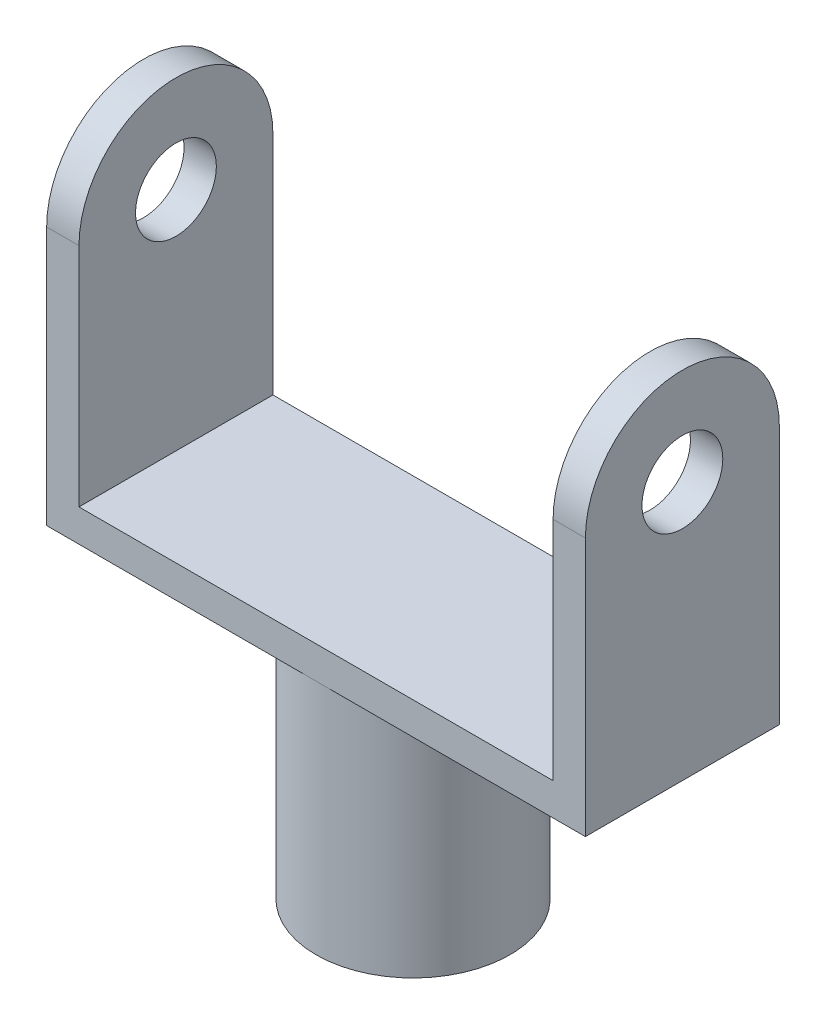
ISO-10303-21;
HEADER;
FILE_DESCRIPTION(('STEP AP214'),'2;1');
FILE_NAME('part.step','',(''),(''),'','','');
FILE_SCHEMA(('AUTOMOTIVE_DESIGN { 1 0 10303 214 1 1 1 1 }'));
ENDSEC;
DATA;
#1=APPLICATION_CONTEXT('core data for automotive mechanical design processes');
#2=APPLICATION_PROTOCOL_DEFINITION('international standard','automotive_design',2000,#1);
#3=PRODUCT_CONTEXT('',#1,'mechanical');
#4=PRODUCT('Part','Part','',(#3));
#5=PRODUCT_RELATED_PRODUCT_CATEGORY('part','',(#4));
#6=PRODUCT_DEFINITION_FORMATION('','',#4);
#7=PRODUCT_DEFINITION_CONTEXT('part definition',#1,'design');
#8=PRODUCT_DEFINITION('design','',#6,#7);
#9=PRODUCT_DEFINITION_SHAPE('','',#8);
#10=(LENGTH_UNIT() NAMED_UNIT(*) SI_UNIT(.MILLI.,.METRE.));
#11=(NAMED_UNIT(*) PLANE_ANGLE_UNIT() SI_UNIT($,.RADIAN.));
#12=(NAMED_UNIT(*) SI_UNIT($,.STERADIAN.) SOLID_ANGLE_UNIT());
#13=UNCERTAINTY_MEASURE_WITH_UNIT(LENGTH_MEASURE(1.E-05),#10,'distance_accuracy_value','');
#14=(GEOMETRIC_REPRESENTATION_CONTEXT(3) GLOBAL_UNCERTAINTY_ASSIGNED_CONTEXT((#13)) GLOBAL_UNIT_ASSIGNED_CONTEXT((#10,
#11,#12)) REPRESENTATION_CONTEXT('',''));
#15=CARTESIAN_POINT('',(0.,0.,0.));
#16=DIRECTION('',(0.,0.,1.));
#17=DIRECTION('',(1.,0.,0.));
#18=AXIS2_PLACEMENT_3D('',#15,#16,#17);
#19=CARTESIAN_POINT('',(0.,44.,0.));
#20=DIRECTION('',(0.,-1.,0.));
#21=DIRECTION('',(0.,0.,-1.));
#22=AXIS2_PLACEMENT_3D('',#19,#20,#21);
#23=CYLINDRICAL_SURFACE('',#22,18.);
#24=CARTESIAN_POINT('',(0.,44.,0.));
#25=DIRECTION('',(0.,1.,0.));
#26=DIRECTION('',(0.,0.,1.));
#27=AXIS2_PLACEMENT_3D('',#24,#25,#26);
#28=CIRCLE('',#27,18.);
#29=CARTESIAN_POINT('',(0.,44.,18.));
#30=VERTEX_POINT('',#29);
#31=CARTESIAN_POINT('',(0.,44.,-18.));
#32=VERTEX_POINT('',#31);
#33=EDGE_CURVE('E11',#30,#32,#28,.T.);
#34=ORIENTED_EDGE('',*,*,#33,.F.);
#35=EDGE_CURVE('E47',#32,#30,#28,.T.);
#36=ORIENTED_EDGE('',*,*,#35,.F.);
#37=EDGE_LOOP('',(#34,#36));
#38=FACE_BOUND('',#37,.T.);
#39=CARTESIAN_POINT('',(0.,0.,0.));
#40=DIRECTION('',(0.,1.,0.));
#41=DIRECTION('',(0.,0.,1.));
#42=AXIS2_PLACEMENT_3D('',#39,#40,#41);
#43=CIRCLE('',#42,18.);
#44=CARTESIAN_POINT('',(0.,0.,18.));
#45=VERTEX_POINT('',#44);
#46=EDGE_CURVE('E42',#45,#45,#43,.T.);
#47=ORIENTED_EDGE('',*,*,#46,.T.);
#48=EDGE_LOOP('',(#47));
#49=FACE_BOUND('',#48,.T.);
#50=ADVANCED_FACE('F41',(#38,#49),#23,.T.);
#51=CARTESIAN_POINT('',(0.,0.,0.));
#52=DIRECTION('',(0.,1.,0.));
#53=DIRECTION('',(0.,0.,1.));
#54=AXIS2_PLACEMENT_3D('',#51,#52,#53);
#55=PLANE('',#54);
#56=ORIENTED_EDGE('',*,*,#46,.F.);
#57=EDGE_LOOP('',(#56));
#58=FACE_BOUND('',#57,.T.);
#59=ADVANCED_FACE('F221',(#58),#55,.F.);
#60=CARTESIAN_POINT('',(0.,44.,0.));
#61=DIRECTION('',(0.,-1.,0.));
#62=DIRECTION('',(0.,0.,-1.));
#63=AXIS2_PLACEMENT_3D('',#60,#61,#62);
#64=PLANE('',#63);
#65=DIRECTION('',(1.,0.,0.));
#66=VECTOR('',#65,1.);
#67=CARTESIAN_POINT('',(-44.,44.,18.));
#68=LINE('',#67,#66);
#69=CARTESIAN_POINT('',(50.,44.,18.));
#70=VERTEX_POINT('',#69);
#71=EDGE_CURVE('E186',#30,#70,#68,.T.);
#72=ORIENTED_EDGE('',*,*,#71,.F.);
#73=ORIENTED_EDGE('',*,*,#33,.T.);
#74=DIRECTION('',(-1.,0.,0.));
#75=VECTOR('',#74,1.);
#76=CARTESIAN_POINT('',(-44.,44.,-18.));
#77=LINE('',#76,#75);
#78=CARTESIAN_POINT('',(50.,44.,-18.));
#79=VERTEX_POINT('',#78);
#80=EDGE_CURVE('E189',#79,#32,#77,.T.);
#81=ORIENTED_EDGE('',*,*,#80,.F.);
#82=DIRECTION('',(0.,0.,-1.));
#83=VECTOR('',#82,1.);
#84=CARTESIAN_POINT('',(50.,44.,18.));
#85=LINE('',#84,#83);
#86=EDGE_CURVE('E152',#70,#79,#85,.T.);
#87=ORIENTED_EDGE('',*,*,#86,.F.);
#88=EDGE_LOOP('',(#72,#73,#81,#87));
#89=FACE_BOUND('',#88,.T.);
#90=ADVANCED_FACE('F192',(#89),#64,.T.);
#91=CARTESIAN_POINT('',(-44.,50.,-18.));
#92=DIRECTION('',(0.,0.,1.));
#93=DIRECTION('',(1.,0.,0.));
#94=AXIS2_PLACEMENT_3D('',#91,#92,#93);
#95=PLANE('',#94);
#96=ORIENTED_EDGE('',*,*,#80,.T.);
#97=CARTESIAN_POINT('',(-50.,44.,-18.));
#98=VERTEX_POINT('',#97);
#99=EDGE_CURVE('E172',#32,#98,#77,.T.);
#100=ORIENTED_EDGE('',*,*,#99,.T.);
#101=DIRECTION('',(0.,1.,0.));
#102=VECTOR('',#101,1.);
#103=CARTESIAN_POINT('',(-50.,44.,-18.));
#104=LINE('',#103,#102);
#105=CARTESIAN_POINT('',(-50.,92.,-18.));
#106=VERTEX_POINT('',#105);
#107=EDGE_CURVE('E132',#98,#106,#104,.T.);
#108=ORIENTED_EDGE('',*,*,#107,.T.);
#109=DIRECTION('',(1.,0.,0.));
#110=VECTOR('',#109,1.);
#111=CARTESIAN_POINT('',(-50.,92.,-18.));
#112=LINE('',#111,#110);
#113=CARTESIAN_POINT('',(-44.,92.,-18.));
#114=VERTEX_POINT('',#113);
#115=EDGE_CURVE('E120',#106,#114,#112,.T.);
#116=ORIENTED_EDGE('',*,*,#115,.T.);
#117=DIRECTION('',(0.,1.,0.));
#118=VECTOR('',#117,1.);
#119=CARTESIAN_POINT('',(-44.,44.,-18.));
#120=LINE('',#119,#118);
#121=CARTESIAN_POINT('',(-44.,50.,-18.));
#122=VERTEX_POINT('',#121);
#123=EDGE_CURVE('E129',#122,#114,#120,.T.);
#124=ORIENTED_EDGE('',*,*,#123,.F.);
#125=DIRECTION('',(-1.,0.,0.));
#126=VECTOR('',#125,1.);
#127=CARTESIAN_POINT('',(-44.,50.,-18.));
#128=LINE('',#127,#126);
#129=CARTESIAN_POINT('',(44.,50.,-18.));
#130=VERTEX_POINT('',#129);
#131=EDGE_CURVE('E180',#130,#122,#128,.T.);
#132=ORIENTED_EDGE('',*,*,#131,.F.);
#133=DIRECTION('',(0.,1.,0.));
#134=VECTOR('',#133,1.);
#135=CARTESIAN_POINT('',(44.,44.,-18.));
#136=LINE('',#135,#134);
#137=CARTESIAN_POINT('',(44.,92.,-18.));
#138=VERTEX_POINT('',#137);
#139=EDGE_CURVE('E164',#130,#138,#136,.T.);
#140=ORIENTED_EDGE('',*,*,#139,.T.);
#141=DIRECTION('',(-1.,0.,0.));
#142=VECTOR('',#141,1.);
#143=CARTESIAN_POINT('',(50.,92.,-18.));
#144=LINE('',#143,#142);
#145=CARTESIAN_POINT('',(50.,92.,-18.));
#146=VERTEX_POINT('',#145);
#147=EDGE_CURVE('E168',#146,#138,#144,.T.);
#148=ORIENTED_EDGE('',*,*,#147,.F.);
#149=DIRECTION('',(0.,1.,0.));
#150=VECTOR('',#149,1.);
#151=CARTESIAN_POINT('',(50.,44.,-18.));
#152=LINE('',#151,#150);
#153=EDGE_CURVE('E158',#79,#146,#152,.T.);
#154=ORIENTED_EDGE('',*,*,#153,.F.);
#155=EDGE_LOOP('',(#96,#100,#108,#116,#124,#132,#140,#148,#154));
#156=FACE_BOUND('',#155,.T.);
#157=ADVANCED_FACE('F216',(#156),#95,.F.);
#158=CARTESIAN_POINT('',(-44.,50.,18.));
#159=DIRECTION('',(0.,0.,-1.));
#160=DIRECTION('',(-1.,0.,0.));
#161=AXIS2_PLACEMENT_3D('',#158,#159,#160);
#162=PLANE('',#161);
#163=CARTESIAN_POINT('',(-50.,44.,18.));
#164=VERTEX_POINT('',#163);
#165=EDGE_CURVE('E176',#164,#30,#68,.T.);
#166=ORIENTED_EDGE('',*,*,#165,.T.);
#167=ORIENTED_EDGE('',*,*,#71,.T.);
#168=DIRECTION('',(0.,-1.,0.));
#169=VECTOR('',#168,1.);
#170=CARTESIAN_POINT('',(50.,44.,18.));
#171=LINE('',#170,#169);
#172=CARTESIAN_POINT('',(50.,92.,18.));
#173=VERTEX_POINT('',#172);
#174=EDGE_CURVE('E151',#173,#70,#171,.T.);
#175=ORIENTED_EDGE('',*,*,#174,.F.);
#176=DIRECTION('',(-1.,0.,0.));
#177=VECTOR('',#176,1.);
#178=CARTESIAN_POINT('',(50.,92.,18.));
#179=LINE('',#178,#177);
#180=CARTESIAN_POINT('',(44.,92.,18.));
#181=VERTEX_POINT('',#180);
#182=EDGE_CURVE('E165',#173,#181,#179,.T.);
#183=ORIENTED_EDGE('',*,*,#182,.T.);
#184=DIRECTION('',(0.,-1.,0.));
#185=VECTOR('',#184,1.);
#186=CARTESIAN_POINT('',(44.,44.,18.));
#187=LINE('',#186,#185);
#188=CARTESIAN_POINT('',(44.,50.,18.));
#189=VERTEX_POINT('',#188);
#190=EDGE_CURVE('E146',#181,#189,#187,.T.);
#191=ORIENTED_EDGE('',*,*,#190,.T.);
#192=DIRECTION('',(1.,0.,0.));
#193=VECTOR('',#192,1.);
#194=CARTESIAN_POINT('',(-44.,50.,18.));
#195=LINE('',#194,#193);
#196=CARTESIAN_POINT('',(-44.,50.,18.));
#197=VERTEX_POINT('',#196);
#198=EDGE_CURVE('E184',#197,#189,#195,.T.);
#199=ORIENTED_EDGE('',*,*,#198,.F.);
#200=DIRECTION('',(0.,-1.,0.));
#201=VECTOR('',#200,1.);
#202=CARTESIAN_POINT('',(-44.,44.,18.));
#203=LINE('',#202,#201);
#204=CARTESIAN_POINT('',(-44.,92.,18.));
#205=VERTEX_POINT('',#204);
#206=EDGE_CURVE('E114',#205,#197,#203,.T.);
#207=ORIENTED_EDGE('',*,*,#206,.F.);
#208=DIRECTION('',(1.,0.,0.));
#209=VECTOR('',#208,1.);
#210=CARTESIAN_POINT('',(-50.,92.,18.));
#211=LINE('',#210,#209);
#212=CARTESIAN_POINT('',(-50.,92.,18.));
#213=VERTEX_POINT('',#212);
#214=EDGE_CURVE('E106',#213,#205,#211,.T.);
#215=ORIENTED_EDGE('',*,*,#214,.F.);
#216=DIRECTION('',(0.,-1.,0.));
#217=VECTOR('',#216,1.);
#218=CARTESIAN_POINT('',(-50.,44.,18.));
#219=LINE('',#218,#217);
#220=EDGE_CURVE('E109',#213,#164,#219,.T.);
#221=ORIENTED_EDGE('',*,*,#220,.T.);
#222=EDGE_LOOP('',(#166,#167,#175,#183,#191,#199,#207,#215,#221));
#223=FACE_BOUND('',#222,.T.);
#224=ADVANCED_FACE('F108',(#223),#162,.F.);
#225=CARTESIAN_POINT('',(0.,50.,0.));
#226=DIRECTION('',(0.,-1.,0.));
#227=DIRECTION('',(0.,0.,-1.));
#228=AXIS2_PLACEMENT_3D('',#225,#226,#227);
#229=PLANE('',#228);
#230=DIRECTION('',(0.,0.,-1.));
#231=VECTOR('',#230,1.);
#232=CARTESIAN_POINT('',(44.,50.,18.));
#233=LINE('',#232,#231);
#234=EDGE_CURVE('E175',#189,#130,#233,.T.);
#235=ORIENTED_EDGE('',*,*,#234,.T.);
#236=ORIENTED_EDGE('',*,*,#131,.T.);
#237=DIRECTION('',(0.,0.,1.));
#238=VECTOR('',#237,1.);
#239=CARTESIAN_POINT('',(-44.,50.,18.));
#240=LINE('',#239,#238);
#241=EDGE_CURVE('E182',#122,#197,#240,.T.);
#242=ORIENTED_EDGE('',*,*,#241,.T.);
#243=ORIENTED_EDGE('',*,*,#198,.T.);
#244=EDGE_LOOP('',(#235,#236,#242,#243));
#245=FACE_BOUND('',#244,.T.);
#246=ADVANCED_FACE('F211',(#245),#229,.F.);
#247=ORIENTED_EDGE('',*,*,#99,.F.);
#248=ORIENTED_EDGE('',*,*,#35,.T.);
#249=ORIENTED_EDGE('',*,*,#165,.F.);
#250=DIRECTION('',(0.,0.,-1.));
#251=VECTOR('',#250,1.);
#252=CARTESIAN_POINT('',(-50.,44.,18.));
#253=LINE('',#252,#251);
#254=EDGE_CURVE('E126',#164,#98,#253,.T.);
#255=ORIENTED_EDGE('',*,*,#254,.T.);
#256=EDGE_LOOP('',(#247,#248,#249,#255));
#257=FACE_BOUND('',#256,.T.);
#258=ADVANCED_FACE('F218',(#257),#64,.T.);
#259=CARTESIAN_POINT('',(44.,92.,0.));
#260=DIRECTION('',(-1.,0.,0.));
#261=DIRECTION('',(0.,0.,1.));
#262=AXIS2_PLACEMENT_3D('',#259,#260,#261);
#263=PLANE('',#262);
#264=CARTESIAN_POINT('',(44.,92.,0.));
#265=DIRECTION('',(1.,0.,0.));
#266=DIRECTION('',(0.,0.,-1.));
#267=AXIS2_PLACEMENT_3D('',#264,#265,#266);
#268=CIRCLE('',#267,7.5);
#269=CARTESIAN_POINT('',(44.,92.,-7.5));
#270=VERTEX_POINT('',#269);
#271=EDGE_CURVE('E117',#270,#270,#268,.T.);
#272=ORIENTED_EDGE('',*,*,#271,.T.);
#273=EDGE_LOOP('',(#272));
#274=FACE_BOUND('',#273,.T.);
#275=ORIENTED_EDGE('',*,*,#234,.F.);
#276=ORIENTED_EDGE('',*,*,#190,.F.);
#277=CARTESIAN_POINT('',(44.,92.,0.));
#278=DIRECTION('',(1.,0.,0.));
#279=DIRECTION('',(0.,0.,1.));
#280=AXIS2_PLACEMENT_3D('',#277,#278,#279);
#281=CIRCLE('',#280,18.);
#282=EDGE_CURVE('E154',#138,#181,#281,.T.);
#283=ORIENTED_EDGE('',*,*,#282,.F.);
#284=ORIENTED_EDGE('',*,*,#139,.F.);
#285=EDGE_LOOP('',(#275,#276,#283,#284));
#286=FACE_BOUND('',#285,.T.);
#287=ADVANCED_FACE('F208',(#274,#286),#263,.T.);
#288=CARTESIAN_POINT('',(50.,92.,0.));
#289=DIRECTION('',(-1.,0.,0.));
#290=DIRECTION('',(0.,0.,1.));
#291=AXIS2_PLACEMENT_3D('',#288,#289,#290);
#292=PLANE('',#291);
#293=ORIENTED_EDGE('',*,*,#174,.T.);
#294=ORIENTED_EDGE('',*,*,#86,.T.);
#295=ORIENTED_EDGE('',*,*,#153,.T.);
#296=CARTESIAN_POINT('',(50.,92.,0.));
#297=DIRECTION('',(1.,0.,0.));
#298=DIRECTION('',(0.,0.,1.));
#299=AXIS2_PLACEMENT_3D('',#296,#297,#298);
#300=CIRCLE('',#299,18.);
#301=EDGE_CURVE('E159',#146,#173,#300,.T.);
#302=ORIENTED_EDGE('',*,*,#301,.T.);
#303=EDGE_LOOP('',(#293,#294,#295,#302));
#304=FACE_BOUND('',#303,.T.);
#305=CARTESIAN_POINT('',(50.,92.,0.));
#306=DIRECTION('',(1.,0.,0.));
#307=DIRECTION('',(0.,0.,-1.));
#308=AXIS2_PLACEMENT_3D('',#305,#306,#307);
#309=CIRCLE('',#308,7.5);
#310=CARTESIAN_POINT('',(50.,92.,-7.5));
#311=VERTEX_POINT('',#310);
#312=EDGE_CURVE('E144',#311,#311,#309,.T.);
#313=ORIENTED_EDGE('',*,*,#312,.F.);
#314=EDGE_LOOP('',(#313));
#315=FACE_BOUND('',#314,.T.);
#316=ADVANCED_FACE('F196',(#304,#315),#292,.F.);
#317=CARTESIAN_POINT('',(50.,92.,0.));
#318=DIRECTION('',(-1.,0.,0.));
#319=DIRECTION('',(0.,0.,1.));
#320=AXIS2_PLACEMENT_3D('',#317,#318,#319);
#321=CYLINDRICAL_SURFACE('',#320,18.);
#322=ORIENTED_EDGE('',*,*,#282,.T.);
#323=ORIENTED_EDGE('',*,*,#182,.F.);
#324=ORIENTED_EDGE('',*,*,#301,.F.);
#325=ORIENTED_EDGE('',*,*,#147,.T.);
#326=EDGE_LOOP('',(#322,#323,#324,#325));
#327=FACE_BOUND('',#326,.T.);
#328=ADVANCED_FACE('F204',(#327),#321,.T.);
#329=CARTESIAN_POINT('',(50.,92.,0.));
#330=DIRECTION('',(-1.,0.,0.));
#331=DIRECTION('',(0.,0.,1.));
#332=AXIS2_PLACEMENT_3D('',#329,#330,#331);
#333=CYLINDRICAL_SURFACE('',#332,7.5);
#334=ORIENTED_EDGE('',*,*,#312,.T.);
#335=EDGE_LOOP('',(#334));
#336=FACE_BOUND('',#335,.T.);
#337=ORIENTED_EDGE('',*,*,#271,.F.);
#338=EDGE_LOOP('',(#337));
#339=FACE_BOUND('',#338,.T.);
#340=ADVANCED_FACE('F243',(#336,#339),#333,.F.);
#341=CARTESIAN_POINT('',(-44.,92.,0.));
#342=DIRECTION('',(1.,0.,0.));
#343=DIRECTION('',(0.,0.,1.));
#344=AXIS2_PLACEMENT_3D('',#341,#342,#343);
#345=PLANE('',#344);
#346=CARTESIAN_POINT('',(-44.,92.,0.));
#347=DIRECTION('',(1.,0.,0.));
#348=DIRECTION('',(0.,0.,-1.));
#349=AXIS2_PLACEMENT_3D('',#346,#347,#348);
#350=CIRCLE('',#349,7.5);
#351=CARTESIAN_POINT('',(-44.,92.,-7.5));
#352=VERTEX_POINT('',#351);
#353=EDGE_CURVE('E268',#352,#352,#350,.T.);
#354=ORIENTED_EDGE('',*,*,#353,.F.);
#355=EDGE_LOOP('',(#354));
#356=FACE_BOUND('',#355,.T.);
#357=ORIENTED_EDGE('',*,*,#241,.F.);
#358=ORIENTED_EDGE('',*,*,#123,.T.);
#359=CARTESIAN_POINT('',(-44.,92.,0.));
#360=DIRECTION('',(1.,0.,0.));
#361=DIRECTION('',(0.,0.,1.));
#362=AXIS2_PLACEMENT_3D('',#359,#360,#361);
#363=CIRCLE('',#362,18.);
#364=EDGE_CURVE('E137',#114,#205,#363,.T.);
#365=ORIENTED_EDGE('',*,*,#364,.T.);
#366=ORIENTED_EDGE('',*,*,#206,.T.);
#367=EDGE_LOOP('',(#357,#358,#365,#366));
#368=FACE_BOUND('',#367,.T.);
#369=ADVANCED_FACE('F212',(#356,#368),#345,.T.);
#370=CARTESIAN_POINT('',(-50.,92.,0.));
#371=DIRECTION('',(1.,0.,0.));
#372=DIRECTION('',(0.,0.,-1.));
#373=AXIS2_PLACEMENT_3D('',#370,#371,#372);
#374=CYLINDRICAL_SURFACE('',#373,18.);
#375=ORIENTED_EDGE('',*,*,#364,.F.);
#376=ORIENTED_EDGE('',*,*,#115,.F.);
#377=CARTESIAN_POINT('',(-50.,92.,0.));
#378=DIRECTION('',(1.,0.,0.));
#379=DIRECTION('',(0.,0.,1.));
#380=AXIS2_PLACEMENT_3D('',#377,#378,#379);
#381=CIRCLE('',#380,18.);
#382=EDGE_CURVE('E122',#106,#213,#381,.T.);
#383=ORIENTED_EDGE('',*,*,#382,.T.);
#384=ORIENTED_EDGE('',*,*,#214,.T.);
#385=EDGE_LOOP('',(#375,#376,#383,#384));
#386=FACE_BOUND('',#385,.T.);
#387=ADVANCED_FACE('F133',(#386),#374,.T.);
#388=CARTESIAN_POINT('',(-50.,92.,0.));
#389=DIRECTION('',(1.,0.,0.));
#390=DIRECTION('',(0.,0.,1.));
#391=AXIS2_PLACEMENT_3D('',#388,#389,#390);
#392=PLANE('',#391);
#393=CARTESIAN_POINT('',(-50.,92.,0.));
#394=DIRECTION('',(1.,0.,0.));
#395=DIRECTION('',(0.,0.,-1.));
#396=AXIS2_PLACEMENT_3D('',#393,#394,#395);
#397=CIRCLE('',#396,7.5);
#398=CARTESIAN_POINT('',(-50.,92.,-7.5));
#399=VERTEX_POINT('',#398);
#400=EDGE_CURVE('E143',#399,#399,#397,.T.);
#401=ORIENTED_EDGE('',*,*,#400,.T.);
#402=EDGE_LOOP('',(#401));
#403=FACE_BOUND('',#402,.T.);
#404=ORIENTED_EDGE('',*,*,#220,.F.);
#405=ORIENTED_EDGE('',*,*,#382,.F.);
#406=ORIENTED_EDGE('',*,*,#107,.F.);
#407=ORIENTED_EDGE('',*,*,#254,.F.);
#408=EDGE_LOOP('',(#404,#405,#406,#407));
#409=FACE_BOUND('',#408,.T.);
#410=ADVANCED_FACE('F121',(#403,#409),#392,.F.);
#411=CARTESIAN_POINT('',(-50.,92.,0.));
#412=DIRECTION('',(1.,0.,0.));
#413=DIRECTION('',(0.,0.,-1.));
#414=AXIS2_PLACEMENT_3D('',#411,#412,#413);
#415=CYLINDRICAL_SURFACE('',#414,7.5);
#416=ORIENTED_EDGE('',*,*,#400,.F.);
#417=EDGE_LOOP('',(#416));
#418=FACE_BOUND('',#417,.T.);
#419=ORIENTED_EDGE('',*,*,#353,.T.);
#420=EDGE_LOOP('',(#419));
#421=FACE_BOUND('',#420,.T.);
#422=ADVANCED_FACE('F260',(#418,#421),#415,.F.);
#423=CLOSED_SHELL('',(#50,#59,#90,#157,#224,#246,#258,#287,#316,#328,#340,#369,#387,#410,#422));
#424=MANIFOLD_SOLID_BREP('B2',#423);
#425=ADVANCED_BREP_SHAPE_REPRESENTATION('',(#18,#424),#14);
#426=SHAPE_DEFINITION_REPRESENTATION(#9,#425);
ENDSEC;
END-ISO-10303-21;
